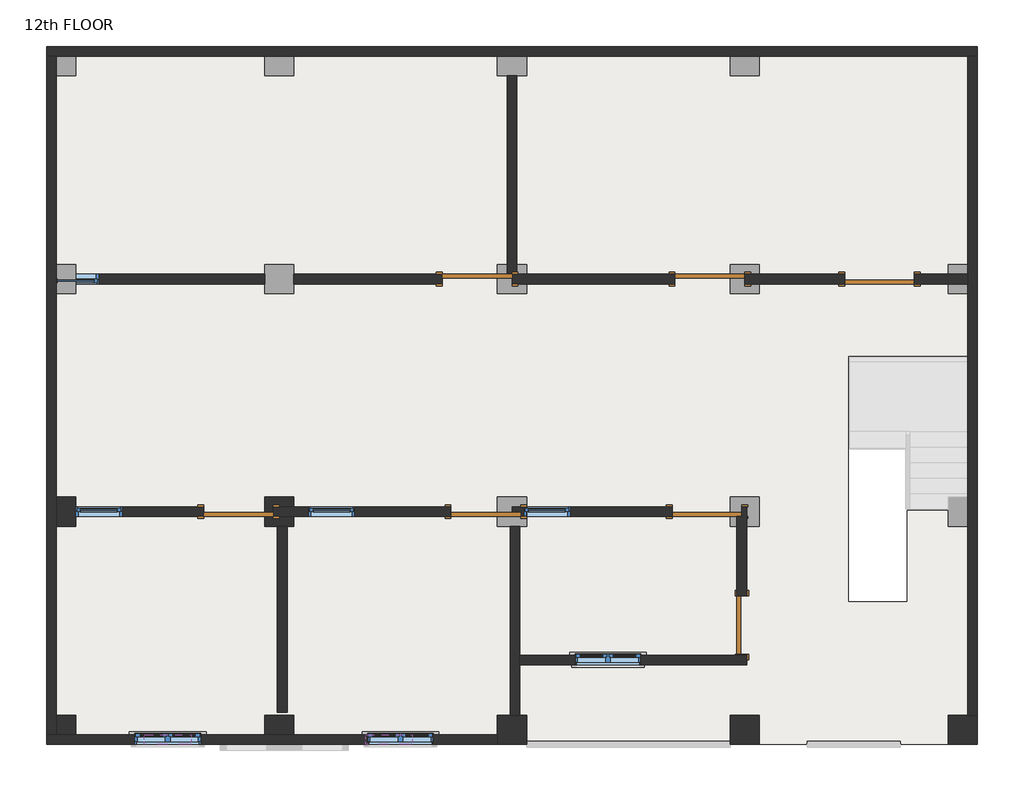
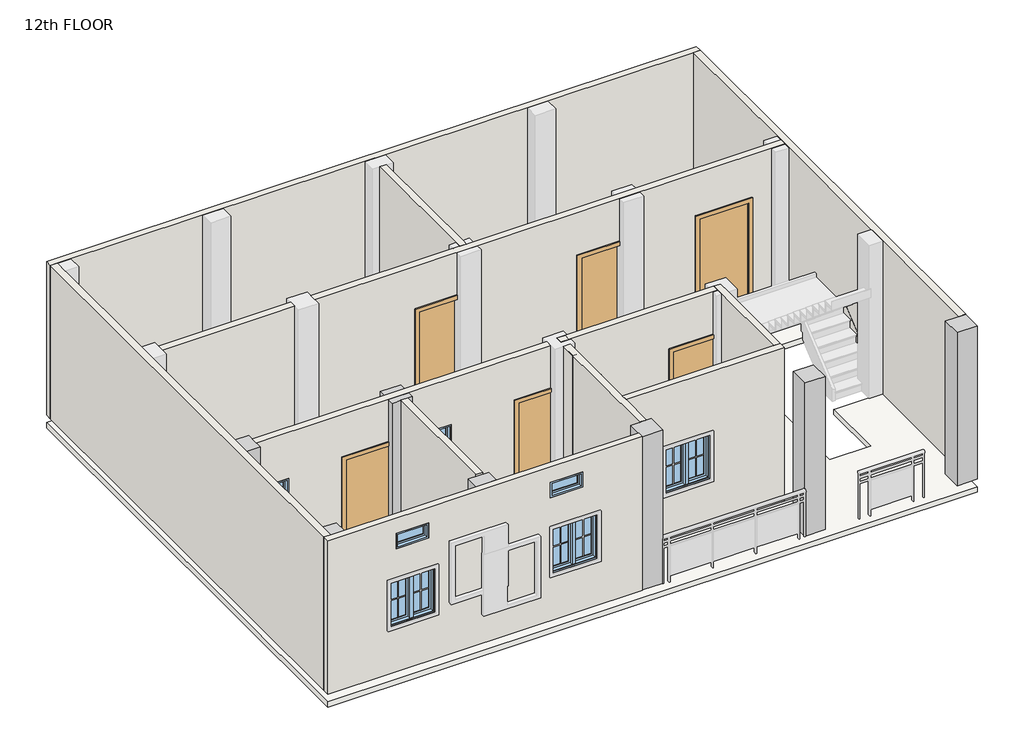
# One storey, part 1 of 2: 15 walls, 9 windows, 7 columns, 7 doors, 1 slab.
"""IFC4 building model written with IfcOpenShell, lengths in millimetres."""

from ifc_helpers import new_model, si_unit, frame, origin, place, context, project, spatial, polyline, outline, extrude, faceted_brep, transform, mapped, element, save
from components import door_e00f436c, door_a1797ceb, window_4c2727af, window_0bf3737e, window_78893e6c, window_0d9958e7

model = new_model("IFC4")

# Units and contexts
model_context = context("Model", 3, world=origin())
ifc_project = project(units=[si_unit("LENGTHUNIT", "METRE", prefix="MILLI")], contexts=[model_context])

# Site, building, storey
site = spatial("IfcSite", under=ifc_project)
building = spatial("IfcBuilding", under=site)
storey = spatial("IfcBuildingStorey", under=building, Name="12th FLOOR", Elevation=36423.6)

# Columns
placement = place(None, origin())
element("IfcColumn", 1, ObjectType="column family : column family", at=placement, inside=storey, context=model_context, shape_type="Brep", body=[
    faceted_brep([(-12576.097125, 2486.2065522, 36428.6), (-12957.097125, 2486.2065522, 36428.6), (-12957.097125, 2867.2065522, 36428.6), (-12576.097125, 2867.2065522, 36428.6), (-12576.097125, 2740.2065522, 36428.6), (-12842.797125, 2740.2065522, 36428.6), (-12842.797125, 2613.2065522, 36428.6), (-12576.097125, 2613.2065522, 36428.6), (-12576.097125, 2486.2065522, 39466.6), (-12576.097125, 2613.2065522, 39466.6), (-12957.097125, 2486.2065522, 39466.6), (-12957.097125, 2613.2065522, 39466.6), (-12957.097125, 2613.2065522, 38557.2), (-12957.097125, 2740.2065522, 38557.2), (-12957.097125, 2740.2065522, 39466.6), (-12957.097125, 2867.2065522, 39466.6), (-12576.097125, 2867.2065522, 39466.6), (-12842.797125, 2613.2065522, 38557.2), (-12842.797125, 2740.2065522, 38557.2), (-12576.097125, 2740.2065522, 39466.6)], [[[0, 1, 2, 3, 4, 5, 6, 7]], [[8, 0, 7, 9]], [[1, 0, 8, 10]], [[2, 1, 10, 11, 12, 13, 14, 15]], [[3, 2, 15, 16]], [[10, 8, 9, 11]], [[6, 17, 12, 11, 9, 7]], [[13, 18, 5, 4, 19, 14]], [[3, 16, 19, 4]], [[16, 15, 14, 19]], [[17, 18, 13, 12]], [[18, 17, 6, 5]]]),
])
element("IfcColumn", 2, ObjectType="column family : column family", at=placement, inside=storey, context=model_context, shape_type="SweptSolid", body=[
    extrude(outline(polyline([(-15433.597125, 2867.2065522), (-15433.597125, 2486.2065522), (-15687.597125, 2486.2065522), (-15687.597125, 2867.2065522), (-15433.597125, 2867.2065522)])), frame((0.0, 0.0, 36428.6), z_axis=(0.0, 0.0, 1.0), x_axis=(1.0, 0.0, 0.0)), (0.0, 0.0, 1.0), 3038.0),
])
element("IfcColumn", 3, ObjectType="column family : column family", at=placement, inside=storey, context=model_context, shape_type="SweptSolid", body=[
    extrude(outline(polyline([(-15433.597125, 9.7065522), (-15433.597125, -244.2934478), (-15687.597125, -244.2934478), (-15687.597125, 9.7065522), (-15433.597125, 9.7065522)])), frame((0.0, 0.0, 36428.6), z_axis=(0.0, 0.0, 1.0), x_axis=(1.0, 0.0, 0.0)), (0.0, 0.0, 1.0), 3038.0),
])
element("IfcColumn", 4, ObjectType="column family : column family", at=placement, inside=storey, context=model_context, shape_type="SweptSolid", body=[
    extrude(outline(polyline([(-3622.597125, 9.7065522), (-3622.597125, -371.2934478), (-4003.597125, -371.2934478), (-4003.597125, 9.7065522), (-3622.597125, 9.7065522)])), frame((0.0, 0.0, 36428.6), z_axis=(0.0, 0.0, 1.0), x_axis=(1.0, 0.0, 0.0)), (0.0, 0.0, 1.0), 3038.0),
])
element("IfcColumn", 5, ObjectType="column family : column family", at=placement, inside=storey, context=model_context, shape_type="SweptSolid", body=[
    extrude(outline(polyline([(-6480.097125, 9.7065522), (-6480.097125, -371.2934478), (-6861.097125, -371.2934478), (-6861.097125, 9.7065522), (-6480.097125, 9.7065522)])), frame((0.0, 0.0, 36428.6), z_axis=(0.0, 0.0, 1.0), x_axis=(1.0, 0.0, 0.0)), (0.0, 0.0, 1.0), 3038.0),
])
element("IfcColumn", 6, ObjectType="column family : column family", at=placement, inside=storey, context=model_context, shape_type="SweptSolid", body=[
    extrude(outline(polyline([(-9528.097125, 9.7065522), (-9528.097125, -371.2934478), (-9909.097125, -371.2934478), (-9909.097125, 9.7065522), (-9528.097125, 9.7065522)])), frame((0.0, 0.0, 36428.6), z_axis=(0.0, 0.0, 1.0), x_axis=(1.0, 0.0, 0.0)), (0.0, 0.0, 1.0), 3038.0),
])
element("IfcColumn", 7, ObjectType="column family : column family", at=placement, inside=storey, context=model_context, shape_type="SweptSolid", body=[
    extrude(outline(polyline([(-12957.097125, 9.7065522), (-12576.097125, 9.7065522), (-12576.097125, -244.2934478), (-12957.097125, -244.2934478), (-12957.097125, 9.7065522)])), frame((0.0, 0.0, 36428.6), z_axis=(0.0, 0.0, 1.0), x_axis=(1.0, 0.0, 0.0)), (0.0, 0.0, 1.0), 3038.0),
])

# Doors
door_shape = door_e00f436c(model_context)
element("IfcDoor", 8, ObjectType="Single-Flush : 30\" x 80\"", at=placement, inside=storey, context=model_context, shape_type="MappedRepresentation", body=[
    mapped(door_shape, transform((-6708.697125, 1190.8065522, 36423.6), x_axis=(0.0, -1.0, 0.0), y_axis=(1.0, 0.0, 0.0), z_axis=(0.0, 0.0, 1.0))),
])
door_2_shape = door_a1797ceb(model_context)
element("IfcDoor", 9, ObjectType="Single-Flush : 36\" x 84\"", at=placement, inside=storey, context=model_context, shape_type="MappedRepresentation", body=[
    mapped(door_2_shape, transform((-10175.797125, 5724.7065522, 36423.6), x_axis=(1.0, 0.0, 0.0), y_axis=(0.0, 1.0, 0.0), z_axis=(0.0, 0.0, 1.0))),
])
element("IfcDoor", 10, ObjectType="Single-Flush : 36\" x 84\"", at=placement, inside=storey, context=model_context, shape_type="MappedRepresentation", body=[
    mapped(door_2_shape, transform((-10061.497125, 2676.7065522, 36423.6), x_axis=(-1.0, 0.0, 0.0), y_axis=(0.0, -1.0, 0.0), z_axis=(0.0, 0.0, 1.0))),
])
element("IfcDoor", 11, ObjectType="Single-Flush : 36\" x 84\"", at=placement, inside=storey, context=model_context, shape_type="MappedRepresentation", body=[
    mapped(door_2_shape, transform((-13299.997125, 2676.7065522, 36423.6), x_axis=(-1.0, 0.0, 0.0), y_axis=(0.0, -1.0, 0.0), z_axis=(0.0, 0.0, 1.0))),
])
element("IfcDoor", 12, ObjectType="Single-Flush : 36\" x 84\"", at=placement, inside=storey, context=model_context, shape_type="MappedRepresentation", body=[
    mapped(door_2_shape, transform((-7127.797125, 5724.7065522, 36423.6), x_axis=(1.0, 0.0, 0.0), y_axis=(0.0, 1.0, 0.0), z_axis=(0.0, 0.0, 1.0))),
])
element("IfcDoor", 13, ObjectType="Single-Flush : 36\" x 84\"", at=placement, inside=storey, context=model_context, shape_type="MappedRepresentation", body=[
    mapped(door_2_shape, transform((-7165.897125, 2676.7065522, 36423.6), x_axis=(-1.0, 0.0, 0.0), y_axis=(0.0, -1.0, 0.0), z_axis=(0.0, 0.0, 1.0))),
])
element("IfcDoor", 14, ObjectType="Single-Flush : 36\" x 84\"", at=placement, inside=storey, context=model_context, shape_type="MappedRepresentation", body=[
    mapped(door_2_shape, transform((-4905.297125, 5724.7065522, 36423.6), x_axis=(-1.0, 0.0, 0.0), y_axis=(0.0, -1.0, 0.0), z_axis=(0.0, 0.0, 1.0))),
])

# Slab
element("IfcSlab", 15, ObjectType="Generic - 4\"", at=placement, inside=storey, context=model_context, shape_type="SweptSolid", body=[
    extrude(outline(polyline([(-3622.597125, 8772.7065522), (-3622.597125, -371.2934478), (-15814.597125, -371.2934478), (-15814.597125, 8772.7065522), (-3622.597125, 8772.7065522)]), holes=[polyline([(-3734.357125, 4711.0719226), (-5310.2646464, 4711.0719226), (-5310.2646464, 1502.3126957), (-4547.7736682, 1502.3126957), (-4547.7736682, 2699.911213), (-3734.357125, 2699.911213), (-3734.357125, 4711.0719226)])]), frame((0.0, 0.0, 36169.6), z_axis=(0.0, 0.0, 1.0), x_axis=(1.0, 0.0, 0.0)), (0.0, 0.0, 1.0), 101.6),
])

# Walls
element("IfcWall", 16, ObjectType="Generic - 5\"", at=placement, inside=storey, context=model_context, shape_type="Brep", body=[
    faceted_brep([(-15814.597125, 8645.7065522, 36423.6), (-15687.597125, 8645.7065522, 36423.6), (-3749.597125, 8645.7065522, 36423.6), (-3622.597125, 8645.7065522, 36423.6), (-3622.597125, 8645.7065522, 39471.6), (-3749.597125, 8645.7065522, 39471.6), (-15687.597125, 8645.7065522, 39471.6), (-15814.597125, 8645.7065522, 39471.6), (-15814.597125, 8772.7065522, 36423.6), (-15814.597125, 8772.7065522, 39471.6), (-3622.597125, 8772.7065522, 39471.6), (-3622.597125, 8772.7065522, 36423.6)], [[[0, 1, 2, 3, 4, 5, 6, 7]], [[8, 9, 10, 11]], [[3, 2, 1, 0, 8, 11]], [[7, 6, 5, 4, 10, 9]], [[4, 3, 11, 10]], [[0, 7, 9, 8]]]),
])
element("IfcWall", 17, ObjectType="Generic - 5\"", at=placement, inside=storey, context=model_context, shape_type="Brep", body=[
    faceted_brep([(-3749.597125, 8645.7065522, 36423.6), (-3749.597125, 5788.2065522, 36423.6), (-3749.597125, 5661.2065522, 36423.6), (-3749.597125, 9.7065522, 36423.6), (-3749.597125, 9.7065522, 39471.6), (-3749.597125, 5661.2065522, 39471.6), (-3749.597125, 5788.2065522, 39471.6), (-3749.597125, 8645.7065522, 39471.6), (-3622.597125, 8645.7065522, 36423.6), (-3622.597125, 8645.7065522, 39471.6), (-3622.597125, 9.7065522, 39471.6), (-3622.597125, 9.7065522, 39466.6), (-3622.597125, 9.7065522, 36428.6), (-3622.597125, 9.7065522, 36423.6)], [[[0, 1, 2, 3, 4, 5, 6, 7]], [[8, 9, 10, 11, 12, 13]], [[3, 2, 1, 0, 8, 13]], [[4, 3, 13, 12, 11, 10]], [[7, 6, 5, 4, 10, 9]], [[0, 7, 9, 8]]]),
])
element("IfcWall", 18, ObjectType="Generic - 5\"", at=placement, inside=storey, context=model_context, shape_type="Brep", body=[
    faceted_brep([(-9909.097125, -244.2934478, 36423.6), (-15687.597125, -244.2934478, 36423.6), (-15814.597125, -244.2934478, 36423.6), (-15814.597125, -244.2934478, 39471.6), (-15687.597125, -244.2934478, 39471.6), (-9909.097125, -244.2934478, 39471.6), (-13795.297125, -244.2934478, 38252.4), (-14658.897125, -244.2934478, 38252.4), (-14658.897125, -244.2934478, 37338.0), (-13795.297125, -244.2934478, 37338.0), (-10747.297125, -244.2934478, 38252.4), (-11610.897125, -244.2934478, 38252.4), (-11610.897125, -244.2934478, 37338.0), (-10747.297125, -244.2934478, 37338.0), (-13922.297125, -244.2934478, 39166.8), (-14531.897125, -244.2934478, 39166.8), (-14531.897125, -244.2934478, 38862.0), (-13922.297125, -244.2934478, 38862.0), (-11026.697125, -244.2934478, 39166.8), (-11636.297125, -244.2934478, 39166.8), (-11636.297125, -244.2934478, 38862.0), (-11026.697125, -244.2934478, 38862.0), (-9909.097125, -371.2934478, 36423.6), (-9909.097125, -371.2934478, 36428.6), (-9909.097125, -371.2934478, 39466.6), (-9909.097125, -371.2934478, 39471.6), (-15814.597125, -371.2934478, 39471.6), (-15814.597125, -371.2934478, 36423.6), (-13795.297125, -371.2934478, 38252.4), (-13795.297125, -371.2934478, 37338.0), (-14658.897125, -371.2934478, 37338.0), (-14658.897125, -371.2934478, 38252.4), (-10747.297125, -371.2934478, 38252.4), (-10747.297125, -371.2934478, 37338.0), (-11610.897125, -371.2934478, 37338.0), (-11610.897125, -371.2934478, 38252.4), (-13922.297125, -371.2934478, 39166.8), (-13922.297125, -371.2934478, 38862.0), (-14531.897125, -371.2934478, 38862.0), (-14531.897125, -371.2934478, 39166.8), (-11026.697125, -371.2934478, 39166.8), (-11026.697125, -371.2934478, 38862.0), (-11636.297125, -371.2934478, 38862.0), (-11636.297125, -371.2934478, 39166.8)], [[[0, 1, 2, 3, 4, 5], [6, 7, 8, 9], [10, 11, 12, 13], [14, 15, 16, 17], [18, 19, 20, 21]], [[22, 23, 24, 25, 26, 27], [28, 29, 30, 31], [32, 33, 34, 35], [36, 37, 38, 39], [40, 41, 42, 43]], [[2, 1, 0, 22, 27]], [[5, 4, 3, 26, 25]], [[0, 5, 25, 24, 23, 22]], [[3, 2, 27, 26]], [[29, 28, 6, 9]], [[30, 29, 9, 8]], [[31, 30, 8, 7]], [[28, 31, 7, 6]], [[33, 32, 10, 13]], [[34, 33, 13, 12]], [[35, 34, 12, 11]], [[32, 35, 11, 10]], [[37, 36, 14, 17]], [[38, 37, 17, 16]], [[39, 38, 16, 15]], [[36, 39, 15, 14]], [[41, 40, 18, 21]], [[42, 41, 21, 20]], [[43, 42, 20, 19]], [[40, 43, 19, 18]]]),
])
element("IfcWall", 19, ObjectType="Generic - 5\"", at=placement, inside=storey, context=model_context, shape_type="Brep", body=[
    faceted_brep([(-15687.597125, -244.2934478, 36423.6), (-15687.597125, 8645.7065522, 36423.6), (-15687.597125, 8645.7065522, 36428.6), (-15687.597125, 8645.7065522, 39466.6), (-15687.597125, 8645.7065522, 39471.6), (-15687.597125, -244.2934478, 39471.6), (-15687.597125, -244.2934478, 39466.6), (-15687.597125, -244.2934478, 36428.6), (-15814.597125, -244.2934478, 36423.6), (-15814.597125, -244.2934478, 39471.6), (-15814.597125, 8645.7065522, 39471.6), (-15814.597125, 8645.7065522, 36423.6)], [[[0, 1, 2, 3, 4, 5, 6, 7]], [[8, 9, 10, 11]], [[1, 0, 8, 11]], [[5, 4, 10, 9]], [[4, 3, 2, 1, 11, 10]], [[0, 7, 6, 5, 9, 8]]]),
])
element("IfcWall", 20, ObjectType="Generic - 5\"", at=placement, inside=storey, context=model_context, shape_type="SweptSolid", body=[
    extrude(outline(polyline([(36423.6, -15433.597125), (36423.6, -12957.097125), (39471.6, -12957.097125), (39471.6, -15433.597125), (38557.2, -15433.597125), (38557.2, -15128.797125), (36728.4, -15128.797125), (36728.4, -15433.597125), (36423.6, -15433.597125)])), frame((0.0, 5661.2065522, 0.0), z_axis=(0.0, 1.0, 0.0), x_axis=(0.0, 0.0, 1.0)), (0.0, 0.0, 1.0), 127.0),
])
element("IfcWall", 21, ObjectType="Generic - 5\"", at=placement, inside=storey, context=model_context, shape_type="Brep", body=[
    faceted_brep([(-9782.097125, 8391.7065522, 36423.6), (-9782.097125, 5788.2065522, 36423.6), (-9782.097125, 5788.2065522, 36428.6), (-9782.097125, 5788.2065522, 38557.2), (-9782.097125, 5788.2065522, 39466.6), (-9782.097125, 5788.2065522, 39471.6), (-9782.097125, 8391.7065522, 39471.6), (-9655.097125, 8391.7065522, 36423.6), (-9655.097125, 8391.7065522, 39471.6), (-9655.097125, 5788.2065522, 39471.6), (-9655.097125, 5788.2065522, 39466.6), (-9655.097125, 5788.2065522, 36428.6), (-9655.097125, 5788.2065522, 36423.6), (-9718.597125, 5788.2065522, 36423.6)], [[[0, 1, 2, 3, 4, 5, 6]], [[7, 8, 9, 10, 11, 12]], [[1, 0, 7, 12, 13]], [[6, 5, 9, 8]], [[0, 6, 8, 7]], [[5, 4, 3, 2, 1, 13, 12, 11, 10, 9]]]),
])
element("IfcWall", 22, ObjectType="Generic - 5\"", at=placement, inside=storey, context=model_context, shape_type="Brep", body=[
    faceted_brep([(-6670.597125, 5661.2065522, 36423.6), (-5362.497125, 5661.2065522, 36423.6), (-5362.497125, 5661.2065522, 38557.2), (-4448.097125, 5661.2065522, 38557.2), (-4448.097125, 5661.2065522, 36423.6), (-3749.597125, 5661.2065522, 36423.6), (-3749.597125, 5661.2065522, 36428.6), (-3749.597125, 5661.2065522, 39466.6), (-3749.597125, 5661.2065522, 39471.6), (-12576.097125, 5661.2065522, 39471.6), (-12576.097125, 5661.2065522, 36423.6), (-10632.997125, 5661.2065522, 36423.6), (-10632.997125, 5661.2065522, 38557.2), (-9909.097125, 5661.2065522, 38557.2), (-9718.597125, 5661.2065522, 38557.2), (-9718.597125, 5661.2065522, 36428.6), (-9718.597125, 5661.2065522, 36423.6), (-7584.997125, 5661.2065522, 36423.6), (-7584.997125, 5661.2065522, 38557.2), (-6861.097125, 5661.2065522, 38557.2), (-6670.597125, 5661.2065522, 38557.2), (-6670.597125, 5661.2065522, 36428.6), (-5362.497125, 5788.2065522, 38557.2), (-5362.497125, 5788.2065522, 36423.6), (-6670.597125, 5788.2065522, 36423.6), (-6670.597125, 5788.2065522, 36428.6), (-6670.597125, 5788.2065522, 38557.2), (-6861.097125, 5788.2065522, 38557.2), (-7584.997125, 5788.2065522, 38557.2), (-7584.997125, 5788.2065522, 36423.6), (-9655.097125, 5788.2065522, 36423.6), (-9718.597125, 5788.2065522, 36423.6), (-9718.597125, 5788.2065522, 36428.6), (-9718.597125, 5788.2065522, 38557.2), (-9782.097125, 5788.2065522, 38557.2), (-9909.097125, 5788.2065522, 38557.2), (-10632.997125, 5788.2065522, 38557.2), (-10632.997125, 5788.2065522, 36423.6), (-12576.097125, 5788.2065522, 36423.6), (-12576.097125, 5788.2065522, 39471.6), (-9782.097125, 5788.2065522, 39471.6), (-9655.097125, 5788.2065522, 39471.6), (-3749.597125, 5788.2065522, 39471.6), (-3749.597125, 5788.2065522, 39466.6), (-3749.597125, 5788.2065522, 36428.6), (-3749.597125, 5788.2065522, 36423.6), (-4448.097125, 5788.2065522, 36423.6), (-4448.097125, 5788.2065522, 38557.2)], [[[0, 1, 2, 3, 4, 5, 6, 7, 8, 9, 10, 11, 12, 13, 14, 15, 16, 17, 18, 19, 20, 21]], [[22, 23, 24, 25, 26, 27, 28, 29, 30, 31, 32, 33, 34, 35, 36, 37, 38, 39, 40, 41, 42, 43, 44, 45, 46, 47]], [[11, 10, 38, 37]], [[17, 16, 31, 30, 29]], [[46, 45, 5, 4]], [[24, 23, 1, 0]], [[9, 8, 42, 41, 40, 39]], [[10, 9, 39, 38]], [[8, 7, 6, 5, 45, 44, 43, 42]], [[33, 32, 31, 16, 15, 14]], [[36, 35, 34, 33, 14, 13, 12]], [[37, 36, 12, 11]], [[26, 25, 24, 0, 21, 20]], [[28, 27, 26, 20, 19, 18]], [[29, 28, 18, 17]], [[2, 1, 23, 22]], [[3, 2, 22, 47]], [[4, 3, 47, 46]]]),
])
element("IfcWall", 23, ObjectType="Generic - 5\"", at=placement, inside=storey, context=model_context, shape_type="Brep", body=[
    faceted_brep([(-14823.997125, 2613.2065522, 36728.4), (-15433.597125, 2613.2065522, 36728.4), (-15433.597125, 2613.2065522, 36423.6), (-13757.197125, 2613.2065522, 36423.6), (-13757.197125, 2613.2065522, 38557.2), (-12957.097125, 2613.2065522, 38557.2), (-12842.797125, 2613.2065522, 38557.2), (-12842.797125, 2613.2065522, 36428.6), (-12842.797125, 2613.2065522, 36423.6), (-10518.697125, 2613.2065522, 36423.6), (-10518.697125, 2613.2065522, 38557.2), (-9909.097125, 2613.2065522, 38557.2), (-9909.097125, 2613.2065522, 39471.6), (-15433.597125, 2613.2065522, 39471.6), (-15433.597125, 2613.2065522, 38557.2), (-14823.997125, 2613.2065522, 38557.2), (-12385.597125, 2613.2065522, 38557.2), (-11775.997125, 2613.2065522, 38557.2), (-11775.997125, 2613.2065522, 36728.4), (-12385.597125, 2613.2065522, 36728.4), (-15433.597125, 2740.2065522, 36423.6), (-15433.597125, 2740.2065522, 36728.4), (-14823.997125, 2740.2065522, 36728.4), (-14823.997125, 2740.2065522, 38557.2), (-15433.597125, 2740.2065522, 38557.2), (-15433.597125, 2740.2065522, 39471.6), (-9909.097125, 2740.2065522, 39471.6), (-9909.097125, 2740.2065522, 38557.2), (-10518.697125, 2740.2065522, 38557.2), (-10518.697125, 2740.2065522, 36423.6), (-12842.797125, 2740.2065522, 36423.6), (-12842.797125, 2740.2065522, 36428.6), (-12842.797125, 2740.2065522, 38557.2), (-12957.097125, 2740.2065522, 38557.2), (-13757.197125, 2740.2065522, 38557.2), (-13757.197125, 2740.2065522, 36423.6), (-12385.597125, 2740.2065522, 38557.2), (-12385.597125, 2740.2065522, 36728.4), (-11775.997125, 2740.2065522, 36728.4), (-11775.997125, 2740.2065522, 38557.2)], [[[0, 1, 2, 3, 4, 5, 6, 7, 8, 9, 10, 11, 12, 13, 14, 15], [16, 17, 18, 19]], [[20, 21, 22, 23, 24, 25, 26, 27, 28, 29, 30, 31, 32, 33, 34, 35], [36, 37, 38, 39]], [[30, 29, 9, 8]], [[20, 35, 3, 2]], [[26, 12, 11, 27]], [[13, 12, 26, 25]], [[14, 13, 25, 24]], [[2, 1, 21, 20]], [[28, 10, 9, 29]], [[10, 28, 27, 11]], [[4, 3, 35, 34]], [[6, 5, 4, 34, 33, 32]], [[8, 7, 6, 32, 31, 30]], [[22, 21, 1, 0]], [[23, 22, 0, 15]], [[24, 23, 15, 14]], [[37, 36, 16, 19]], [[38, 37, 19, 18]], [[39, 38, 18, 17]], [[36, 39, 17, 16]]]),
])
element("IfcWall", 24, ObjectType="Generic - 5\"", at=placement, inside=storey, context=model_context, shape_type="Brep", body=[
    faceted_brep([(-9616.997125, 9.7065522, 36423.6), (-9616.997125, 670.1065522, 36423.6), (-9616.997125, 797.1065522, 36423.6), (-9616.997125, 2486.2065522, 36423.6), (-9616.997125, 2486.2065522, 39471.6), (-9616.997125, 797.1065522, 39471.6), (-9616.997125, 670.1065522, 39471.6), (-9616.997125, 9.7065522, 39471.6), (-9743.997125, 9.7065522, 36423.6), (-9743.997125, 9.7065522, 39471.6), (-9743.997125, 2486.2065522, 39471.6), (-9743.997125, 2486.2065522, 36423.6)], [[[0, 1, 2, 3, 4, 5, 6, 7]], [[8, 9, 10, 11]], [[3, 2, 1, 0, 8, 11]], [[4, 3, 11, 10]], [[7, 6, 5, 4, 10, 9]], [[0, 7, 9, 8]]]),
])
element("IfcWall", 25, ObjectType="Generic - 5\"", at=placement, inside=storey, context=model_context, shape_type="SweptSolid", body=[
    extrude(outline(polyline([(-9743.997125, 2181.4065522), (-9743.997125, 2486.2065522), (-9616.997125, 2486.2065522), (-9616.997125, 2181.4065522), (-9743.997125, 2181.4065522)])), frame((0.0, 0.0, 36423.6), z_axis=(0.0, 0.0, 1.0), x_axis=(1.0, 0.0, 0.0)), (0.0, 0.0, 1.0), 3048.0),
])
element("IfcWall", 26, ObjectType="Generic - 5\"", at=placement, inside=storey, context=model_context, shape_type="Brep", body=[
    faceted_brep([(-6772.197125, 2613.2065522, 39471.6), (-9718.597125, 2613.2065522, 39471.6), (-9718.597125, 2613.2065522, 39466.6), (-9718.597125, 2613.2065522, 36428.6), (-9718.597125, 2613.2065522, 36423.6), (-7623.097125, 2613.2065522, 36423.6), (-7623.097125, 2613.2065522, 38557.2), (-6861.097125, 2613.2065522, 38557.2), (-6772.197125, 2613.2065522, 38557.2), (-6772.197125, 2613.2065522, 39466.6), (-9566.197125, 2613.2065522, 38557.2), (-9528.097125, 2613.2065522, 38557.2), (-8956.597125, 2613.2065522, 38557.2), (-8956.597125, 2613.2065522, 36728.4), (-9528.097125, 2613.2065522, 36728.4), (-9566.197125, 2613.2065522, 36728.4), (-9718.597125, 2740.2065522, 39471.6), (-6772.197125, 2740.2065522, 39471.6), (-6772.197125, 2740.2065522, 38557.2), (-6861.097125, 2740.2065522, 38557.2), (-7623.097125, 2740.2065522, 38557.2), (-7623.097125, 2740.2065522, 36423.6), (-9718.597125, 2740.2065522, 36423.6), (-9718.597125, 2740.2065522, 36428.6), (-9718.597125, 2740.2065522, 39466.6), (-9566.197125, 2740.2065522, 38557.2), (-9566.197125, 2740.2065522, 36728.4), (-9528.097125, 2740.2065522, 36728.4), (-8956.597125, 2740.2065522, 36728.4), (-8956.597125, 2740.2065522, 38557.2), (-9528.097125, 2740.2065522, 38557.2)], [[[0, 1, 2, 3, 4, 5, 6, 7, 8, 9], [10, 11, 12, 13, 14, 15]], [[16, 17, 18, 19, 20, 21, 22, 23, 24], [25, 26, 27, 28, 29, 30]], [[4, 22, 21, 5]], [[1, 0, 17, 16]], [[4, 3, 2, 1, 16, 24, 23, 22]], [[26, 25, 10, 15]], [[28, 27, 26, 15, 14, 13]], [[29, 28, 13, 12]], [[25, 30, 29, 12, 11, 10]], [[20, 6, 5, 21]], [[6, 20, 19, 18, 8, 7]], [[17, 0, 9, 8, 18]]]),
])
element("IfcWall", 27, ObjectType="Generic - 5\"", at=placement, inside=storey, context=model_context, shape_type="Brep", body=[
    faceted_brep([(-6645.197125, 797.1065522, 36423.6), (-6645.197125, 809.8065522, 36423.6), (-6645.197125, 809.8065522, 38455.6), (-6645.197125, 1571.8065522, 38455.6), (-6645.197125, 1571.8065522, 36423.6), (-6645.197125, 2740.2065522, 36423.6), (-6645.197125, 2740.2065522, 36428.6), (-6645.197125, 2740.2065522, 39466.6), (-6645.197125, 2740.2065522, 39471.6), (-6645.197125, 797.1065522, 39471.6), (-6772.197125, 809.8065522, 38455.6), (-6772.197125, 809.8065522, 36423.6), (-6772.197125, 797.1065522, 36423.6), (-6772.197125, 797.1065522, 39471.6), (-6772.197125, 2613.2065522, 39471.6), (-6772.197125, 2740.2065522, 39471.6), (-6772.197125, 2740.2065522, 38557.2), (-6772.197125, 2613.2065522, 38557.2), (-6772.197125, 2613.2065522, 36428.6), (-6772.197125, 2613.2065522, 36423.6), (-6772.197125, 1571.8065522, 36423.6), (-6772.197125, 1571.8065522, 38455.6), (-6708.697125, 2613.2065522, 36423.6), (-6708.697125, 2740.2065522, 36423.6), (-6708.697125, 2613.2065522, 38557.2), (-6708.697125, 2613.2065522, 36428.6), (-6708.697125, 2740.2065522, 38557.2), (-6708.697125, 2740.2065522, 36428.6)], [[[0, 1, 2, 3, 4, 5, 6, 7, 8, 9]], [[10, 11, 12, 13, 14, 15, 16, 17, 18, 19, 20, 21]], [[20, 19, 22, 23, 5, 4]], [[12, 11, 1, 0]], [[9, 8, 15, 14, 13]], [[24, 25, 22, 19, 18, 17]], [[26, 24, 17, 16]], [[22, 25, 24, 26, 27, 23]], [[8, 7, 6, 5, 23, 27, 26, 16, 15]], [[0, 9, 13, 12]], [[2, 1, 11, 10]], [[3, 2, 10, 21]], [[4, 3, 21, 20]]]),
])
element("IfcWall", 28, ObjectType="Generic - 5\"", at=placement, inside=storey, context=model_context, shape_type="Brep", body=[
    faceted_brep([(-9718.597125, 2613.2065522, 36423.6), (-9566.197125, 2613.2065522, 36423.6), (-9566.197125, 2613.2065522, 36728.4), (-9566.197125, 2613.2065522, 38557.2), (-9566.197125, 2613.2065522, 39471.6), (-9718.597125, 2613.2065522, 39471.6), (-9718.597125, 2613.2065522, 39466.6), (-9718.597125, 2613.2065522, 36428.6), (-9718.597125, 2740.2065522, 36423.6), (-9718.597125, 2740.2065522, 36428.6), (-9718.597125, 2740.2065522, 39466.6), (-9718.597125, 2740.2065522, 39471.6), (-9566.197125, 2740.2065522, 39471.6), (-9566.197125, 2740.2065522, 38557.2), (-9566.197125, 2740.2065522, 36728.4), (-9566.197125, 2740.2065522, 36423.6)], [[[0, 1, 2, 3, 4, 5, 6, 7]], [[8, 9, 10, 11, 12, 13, 14, 15]], [[1, 0, 8, 15]], [[4, 3, 2, 1, 15, 14, 13, 12]], [[5, 4, 12, 11]], [[0, 7, 6, 5, 11, 10, 9, 8]]]),
])
element("IfcWall", 29, ObjectType="Generic - 5\"", at=placement, inside=storey, context=model_context, shape_type="SweptSolid", body=[
    extrude(outline(polyline([(-12791.997125, 47.8065522), (-12791.997125, 2486.2065522), (-12664.997125, 2486.2065522), (-12664.997125, 47.8065522), (-12791.997125, 47.8065522)])), frame((0.0, 0.0, 36423.6), z_axis=(0.0, 0.0, 1.0), x_axis=(1.0, 0.0, 0.0)), (0.0, 0.0, 1.0), 3048.0),
])
element("IfcWall", 30, ObjectType="Generic - 5\"", at=placement, inside=storey, context=model_context, shape_type="Brep", body=[
    faceted_brep([(-9616.997125, 670.1065522, 36423.6), (-6645.197125, 670.1065522, 36423.6), (-6645.197125, 670.1065522, 39471.6), (-9616.997125, 670.1065522, 39471.6), (-8029.497125, 670.1065522, 38252.4), (-8029.497125, 670.1065522, 37338.0), (-8893.097125, 670.1065522, 37338.0), (-8893.097125, 670.1065522, 38252.4), (-9616.997125, 797.1065522, 36423.6), (-9616.997125, 797.1065522, 39471.6), (-6772.197125, 797.1065522, 39471.6), (-6645.197125, 797.1065522, 39471.6), (-6645.197125, 797.1065522, 36423.6), (-6772.197125, 797.1065522, 36423.6), (-8029.497125, 797.1065522, 38252.4), (-8893.097125, 797.1065522, 38252.4), (-8893.097125, 797.1065522, 37338.0), (-8029.497125, 797.1065522, 37338.0)], [[[0, 1, 2, 3], [4, 5, 6, 7]], [[8, 9, 10, 11, 12, 13], [14, 15, 16, 17]], [[1, 0, 8, 13, 12]], [[3, 2, 11, 10, 9]], [[0, 3, 9, 8]], [[2, 1, 12, 11]], [[5, 4, 14, 17]], [[6, 5, 17, 16]], [[7, 6, 16, 15]], [[4, 7, 15, 14]]]),
])

# Windows
window_shape = window_4c2727af(model_context)
element("IfcWindow", 31, ObjectType="Fixed : 24\" x 12\"", at=placement, inside=storey, context=model_context, shape_type="MappedRepresentation", body=[
    mapped(window_shape, transform((-14188.997125, -307.7934478, 37947.6), x_axis=(1.0, 0.0, 0.0), y_axis=(0.0, 1.0, 0.0), z_axis=(0.0, 0.0, 1.0))),
])
element("IfcWindow", 32, ObjectType="Fixed : 24\" x 12\"", at=placement, inside=storey, context=model_context, shape_type="MappedRepresentation", body=[
    mapped(window_shape, transform((-11293.397125, -307.7934478, 37947.6), x_axis=(1.0, 0.0, 0.0), y_axis=(0.0, 1.0, 0.0), z_axis=(0.0, 0.0, 1.0))),
])
window_2_shape = window_0bf3737e(model_context)
element("IfcWindow", 33, ObjectType="Fixed : 24\" x 72\"", at=placement, inside=storey, context=model_context, shape_type="MappedRepresentation", body=[
    mapped(window_2_shape, transform((-15471.697125, 5724.7065522, 36423.6), x_axis=(-1.0, 0.0, 0.0), y_axis=(0.0, -1.0, 0.0), z_axis=(0.0, 0.0, 1.0))),
])
window_3_shape = window_78893e6c(model_context)
element("IfcWindow", 34, ObjectType="Fixed : 24\" x 72\"", at=placement, inside=storey, context=model_context, shape_type="MappedRepresentation", body=[
    mapped(window_3_shape, transform((-15166.897125, 2676.7065522, 36423.6), x_axis=(-1.0, 0.0, 0.0), y_axis=(0.0, -1.0, 0.0), z_axis=(0.0, 0.0, 1.0))),
])
element("IfcWindow", 35, ObjectType="Fixed : 24\" x 72\"", at=placement, inside=storey, context=model_context, shape_type="MappedRepresentation", body=[
    mapped(window_3_shape, transform((-12118.897125, 2676.7065522, 36423.6), x_axis=(-1.0, 0.0, 0.0), y_axis=(0.0, -1.0, 0.0), z_axis=(0.0, 0.0, 1.0))),
])
element("IfcWindow", 36, ObjectType="Fixed : 24\" x 72\"", at=placement, inside=storey, context=model_context, shape_type="MappedRepresentation", body=[
    mapped(window_3_shape, transform((-9299.497125, 2676.7065522, 36423.6), x_axis=(-1.0, 0.0, 0.0), y_axis=(0.0, -1.0, 0.0), z_axis=(0.0, 0.0, 1.0))),
])
window_4_shape = window_0d9958e7(model_context)
element("IfcWindow", 37, ObjectType="Window-Casement-Double : 34\" x 36\"", at=placement, inside=storey, context=model_context, shape_type="MappedRepresentation", body=[
    mapped(window_4_shape, transform((-14227.097125, -307.7934478, 36423.6), x_axis=(1.0, 0.0, 0.0), y_axis=(0.0, 1.0, 0.0), z_axis=(0.0, 0.0, 1.0))),
])
element("IfcWindow", 38, ObjectType="Window-Casement-Double : 34\" x 36\"", at=placement, inside=storey, context=model_context, shape_type="MappedRepresentation", body=[
    mapped(window_4_shape, transform((-11179.097125, -307.7934478, 36423.6), x_axis=(1.0, 0.0, 0.0), y_axis=(0.0, 1.0, 0.0), z_axis=(0.0, 0.0, 1.0))),
])
element("IfcWindow", 39, ObjectType="Window-Casement-Double : 34\" x 36\"", at=placement, inside=storey, context=model_context, shape_type="MappedRepresentation", body=[
    mapped(window_4_shape, transform((-8461.297125, 733.6065522, 36423.6), x_axis=(1.0, 0.0, 0.0), y_axis=(0.0, 1.0, 0.0), z_axis=(0.0, 0.0, 1.0))),
])

save(model, "model.ifc")

# Revit data of these elements
# Type "column family : column family"
#   w2 [instance default] = 0' - 9.88189"
#   w1 [instance default] = 0' - 9.01575"
#   Depth = 1' - 11.62205"
#   Width = 1' - 11.62205"
# Type "Single-Flush : 30\" x 80\""
#   Type Mark = "5"
#   Construction Type Id = "MDOOR"
#   Assembly Code = "C1020"
#   Analytic Construction = "Metal"
#   Thickness = 0' - 2"
#   Heat Transfer Coefficient (U) = 0.651978 BTU/(h·ft²·°F)
#   Height = 6' - 8"
#   Trim Projection Ext = 0' - 1"
#   Trim Projection Int = 0' - 1"
#   Trim Width = 0' - 3"
#   Width = 2' - 6"
#   Define Thermal Properties by = 1
#   Define Thermal Properties by = 1
#   Door Material = Door - Panel
#   Frame Material = Door - Frame
#   Visual Light Transmittance = 0
#   Solar Heat Gain Coefficient = 0
#   Function = (empty or 0)
#   Wall Closure = (empty or 0)
# Type "Single-Flush : 36\" x 84\""
#   Type Mark = "1"
#   Construction Type Id = "MDOOR"
#   Assembly Code = "C1020"
#   Analytic Construction = "Metal"
#   Thickness = 0' - 2"
#   Heat Transfer Coefficient (U) = 0.651978 BTU/(h·ft²·°F)
#   Height = 7' - 0"
#   Trim Projection Ext = 0' - 1"
#   Trim Projection Int = 0' - 1"
#   Trim Width = 0' - 3"
#   Width = 3' - 0"
#   Define Thermal Properties by = 1
#   Define Thermal Properties by = 1
#   Door Material = Door - Panel
#   Frame Material = Door - Frame
#   Visual Light Transmittance = 0
#   Solar Heat Gain Coefficient = 0
#   Function = (empty or 0)
#   Wall Closure = (empty or 0)
# Type "Generic - 4\""
#   Assembly Code = "B1010"
#   Function = 0
#   Layers, outside or top first: 0' - 4" no material (function 1)
# Type "Generic - 5\""
#   Assembly Code = "B2010"
#   Layers, outside or top first: 0' - 5" no material (function 1)
# Type "Fixed : 24\" x 12\""
#   Type Mark = "4"
#   Construction Type Id = "GSP4R"
#   Assembly Code = "B2020100"
#   Analytic Construction = "1/8 in Pilkington single glazing"
#   Visual Light Transmittance = 0.9
#   Solar Heat Gain Coefficient = 0.78
#   Heat Transfer Coefficient (U) = 0.6496 BTU/(h·ft²·°F)
#   Height = 1' - 0"
#   Default Sill Height = 3' - 0"
#   Width = 2' - 0"
#   Window Inset = 0' - 0 3/4"
#   Define Thermal Properties by = 1
#   Define Thermal Properties by = 1
#   Glass Pane Material = Glass
#   Sash Material = Sash
#   Wall Closure = (empty or 0)
# Type "Fixed : 24\" x 72\""
#   Type Mark = "7"
#   Construction Type Id = "GSP4R"
#   Assembly Code = "B2020100"
#   Analytic Construction = "1/8 in Pilkington single glazing"
#   Visual Light Transmittance = 0.9
#   Solar Heat Gain Coefficient = 0.78
#   Heat Transfer Coefficient (U) = 0.6496 BTU/(h·ft²·°F)
#   Height = 6' - 0"
#   Default Sill Height = 1' - 0"
#   Width = 2' - 0"
#   Window Inset = 0' - 0 3/4"
#   Define Thermal Properties by = 1
#   Define Thermal Properties by = 1
#   Glass Pane Material = Glass
#   Sash Material = Sash
#   Wall Closure = (empty or 0)
# Type "Window-Casement-Double : 34\" x 36\""
#   Type Mark = "14"
#   Fire Rating = "0.5h"
#   Assembly Code = "B2020100"
#   Analytic Construction = "Double glazing - domestic"
#   Frame Extension [instance default] = 0' - 0 1/4"
#   Window Inset [instance default] = 0' - 0"
#   Wall Thickness [instance default] = 0' - 6"
#   Interior Wall Closure [instance default] = 0' - 2 1/4"
#   Half Width = 1' - 5"
#   Visual Light Transmittance = 0.81
#   Thermal Resistance (R) = 1.8146 (h·ft²·°F)/BTU
#   Solar Heat Gain Coefficient = 0.76
#   Rough Width = 2' - 10 1/2"
#   Rough Height = 3' - 0 1/2"
#   Height = 3' - 0"
#   Heat Transfer Coefficient (U) = 0.5511 BTU/(h·ft²·°F)
#   Exterior Wall Closure [instance default] = 0' - 1 1/4"
#   Extension Jamb [instance default] = 0' - 2 1/4"
#   Default Sill Height = 3' - 0"
#   Width = 2' - 10"
#   Define Thermal Properties by = 0
#   Muntin Visibility = yes
#   Interior Trim Visibility [instance default] = yes
#   Exterior Trim Visibility [instance default] = yes
#   Extension Jamb Visibility [instance default] = yes
#   Interior Trim Material = Wood - Stained
#   Muntin Pattern = Muntin Pattern_2x2 : Muntin Pattern_2x2
#   Interior Trim = Trim-Window-Interior-Flat : Picture Frame
#   Interior Frame Material = Wood - Stained
#   Glass Panel Material = Glass
#   Exterior Trim Material = Clad - White
#   Exterior Trim = Trim-Window-Exterior-Flat : with Sill
#   Exterior Frame Material = Clad - White
#   Wall Closure = (empty or 0)
# Element 1 (IfcColumn, "column family : column family")
#   w2 = 1' - 3"
#   w1 = 1' - 3"
#   Phase Created = New Construction
#   Materials on its faces: "Default Wall", "inside wall"
# Element 2 (IfcColumn, "column family : column family")
#   w2 = 1' - 3"
#   w1 = 0' - 10"
#   Phase Created = New Construction
#   Materials on its faces: "inside wall", "Default Wall"
# Elements 3, 7 (IfcColumn, "column family : column family")
#   w2 = 1' - 3"
#   w1 = 1' - 3"
#   Phase Created = New Construction
#   Materials on its faces: "Default Wall"
# Element 4 (IfcColumn, "column family : column family")
#   w2 = 1' - 3"
#   w1 = 1' - 3"
#   Phase Created = New Construction
#   Materials on its faces: "Clad - White", "Default Wall"
# Element 5 (IfcColumn, "column family : column family")
#   w2 = 1' - 3"
#   w1 = 1' - 3"
#   Phase Created = New Construction
#   Materials on its faces: "out side wall"
# Element 6 (IfcColumn, "column family : column family")
#   w2 = 1' - 3"
#   w1 = 1' - 3"
#   Phase Created = New Construction
#   Materials on its faces: "out side wall", "Default Wall"
# Element 8 (IfcDoor, "Single-Flush : 30\" x 80\"")
#   Phase Created = New Construction
#   Materials on its faces: "Door - Frame", "Door - Panel"
# Elements 9, 10, 11, 12, 13, 14 (IfcDoor, "Single-Flush : 36\" x 84\"")
#   Phase Created = New Construction
#   Materials on its faces: "Door - Frame", "Door - Panel"
# Element 15 (IfcSlab, "Generic - 4\"")
#   Height Offset From Level = -0' - 6"
#   Phase Created = New Construction
#   Materials on its faces: "Default Floor", "Clad - White", "floor"
# Element 16 (IfcWall, "Generic - 5\"")
#   Top Offset = 0' - 0"
#   Base Offset = 0' - 0"
#   wall height = 10' - 0"
#   Phase Created = New Construction
#   Base Constraint = 12th FLOOR
#   Top Constraint = 13th FLOOR
#   Materials on its faces: "Default Wall", "Clad - White"
# Element 17 (IfcWall, "Generic - 5\"")
#   Top Offset = 0' - 0"
#   Base Offset = 0' - 0"
#   wall height = 10' - 0"
#   Phase Created = New Construction
#   Base Constraint = 12th FLOOR
#   Top Constraint = 13th FLOOR
#   Materials on its faces: "Default Wall", "grey", "Clad - White"
# Element 18 (IfcWall, "Generic - 5\"")
#   Top Offset = 0' - 0"
#   Base Offset = 0' - 0"
#   wall height = 10' - 0"
#   Phase Created = New Construction
#   Base Constraint = 12th FLOOR
#   Top Constraint = 13th FLOOR
#   Materials on its faces: "Default Wall", "out side wall", "Clad - White"
# Element 19 (IfcWall, "Generic - 5\"")
#   Top Offset = 0' - 0"
#   Base Offset = 0' - 0"
#   wall height = 10' - 0"
#   Phase Created = New Construction
#   Base Constraint = 12th FLOOR
#   Top Constraint = 13th FLOOR
#   Materials on its faces: "Default Wall", "inside wall", "Clad - White"
# Elements 20, 23, 26 (IfcWall, "Generic - 5\"")
#   Top Offset = 0' - 0"
#   Base Offset = 0' - 0"
#   wall height = 10' - 0"
#   Phase Created = New Construction
#   Base Constraint = 12th FLOOR
#   Top Constraint = 13th FLOOR
#   Materials on its faces: "Default Wall", "inside wall"
# Elements 21, 25, 28, 29 (IfcWall, "Generic - 5\"")
#   Top Offset = 0' - 0"
#   Base Offset = 0' - 0"
#   wall height = 10' - 0"
#   Phase Created = New Construction
#   Base Constraint = 12th FLOOR
#   Top Constraint = 13th FLOOR
#   Materials on its faces: "Default Wall"
# Elements 22, 24, 30 (IfcWall, "Generic - 5\"")
#   Top Offset = 0' - 0"
#   Base Offset = 0' - 0"
#   wall height = 10' - 0"
#   Phase Created = New Construction
#   Base Constraint = 12th FLOOR
#   Top Constraint = 13th FLOOR
#   Materials on its faces: "Default Wall", "grey"
# Element 27 (IfcWall, "Generic - 5\"")
#   Top Offset = 0' - 0"
#   Base Offset = 0' - 0"
#   wall height = 10' - 0"
#   Phase Created = New Construction
#   Base Constraint = 12th FLOOR
#   Top Constraint = 13th FLOOR
#   Materials on its faces: "Default Wall", "grey", "inside wall"
# Element 31 (IfcWindow, "Fixed : 24\" x 12\"")
#   Mark = "115"
#   Phase Created = New Construction
#   Materials on its faces: "Sash", "Glass"
# Element 32 (IfcWindow, "Fixed : 24\" x 12\"")
#   Mark = "116"
#   Phase Created = New Construction
#   Materials on its faces: "Sash", "Glass"
# Element 33 (IfcWindow, "Fixed : 24\" x 72\"")
#   Mark = "109"
#   Phase Created = New Construction
#   Materials on its faces: "Sash", "Glass"
# Element 34 (IfcWindow, "Fixed : 24\" x 72\"")
#   Mark = "110"
#   Phase Created = New Construction
#   Materials on its faces: "Sash", "Glass"
# Element 35 (IfcWindow, "Fixed : 24\" x 72\"")
#   Mark = "111"
#   Phase Created = New Construction
#   Materials on its faces: "Sash", "Glass"
# Element 36 (IfcWindow, "Fixed : 24\" x 72\"")
#   Mark = "112"
#   Phase Created = New Construction
#   Materials on its faces: "Sash", "Glass"
# Element 37 (IfcWindow, "Window-Casement-Double : 34\" x 36\"")
#   Mark = "113"
#   Window Inset = 0' - 0"
#   Interior Wall Closure = 0' - 2 1/4"
#   Frame Extension = 0' - 0 1/4"
#   Exterior Wall Closure = 0' - 1 1/4"
#   Interior Trim Visibility = yes
#   Exterior Trim Visibility = yes
#   Phase Created = New Construction
#   Materials on its faces: "Wood - Stained", "Glass", "Clad - White"
# Element 38 (IfcWindow, "Window-Casement-Double : 34\" x 36\"")
#   Mark = "114"
#   Window Inset = 0' - 0"
#   Interior Wall Closure = 0' - 2 1/4"
#   Frame Extension = 0' - 0 1/4"
#   Exterior Wall Closure = 0' - 1 1/4"
#   Interior Trim Visibility = yes
#   Exterior Trim Visibility = yes
#   Phase Created = New Construction
#   Materials on its faces: "Wood - Stained", "Glass", "Clad - White"
# Element 39 (IfcWindow, "Window-Casement-Double : 34\" x 36\"")
#   Mark = "117"
#   Window Inset = 0' - 0"
#   Interior Wall Closure = 0' - 2 1/4"
#   Frame Extension = 0' - 0 1/4"
#   Exterior Wall Closure = 0' - 1 1/4"
#   Interior Trim Visibility = yes
#   Exterior Trim Visibility = yes
#   Phase Created = New Construction
#   Materials on its faces: "Wood - Stained", "Glass", "Clad - White"
# Materials
#   "Door - Panel": class "Wood", colour RGB 210 159 95, transparency 0, Cost = 0
#   "Door - Frame": colour RGB 118 70 51, transparency 0, Cost = 0
#   "Glass": class "Glass", colour RGB 0 128 192, transparency 0.75, Description = "Soda Lime Glass", Cost = 0
#   "Sash": class "Wood", colour RGB 224 178 126, transparency 0, Cost = 0
#   "Wood - Stained": class "Wood", colour RGB 224 178 126, transparency 0, Cost = 0
#   "Clad - White": class "Wood", colour RGB 242 242 238, transparency 0, Cost = 0
#   "Default Wall": colour RGB 128 128 128, transparency 0, Cost = 0
#   "inside wall": class "Generic", colour RGB 199 224 95, transparency 0, Cost = 0
#   "out side wall": class "Generic", colour RGB 16 106 159, transparency 0, Cost = 0
#   "Default Floor": colour RGB 128 128 128, transparency 0, Cost = 0
#   "floor": class "Generic", colour RGB 255 255 255, transparency 0, Cost = 0
#   "grey": class "Generic", colour RGB 80 80 80, transparency 0, Cost = 0
